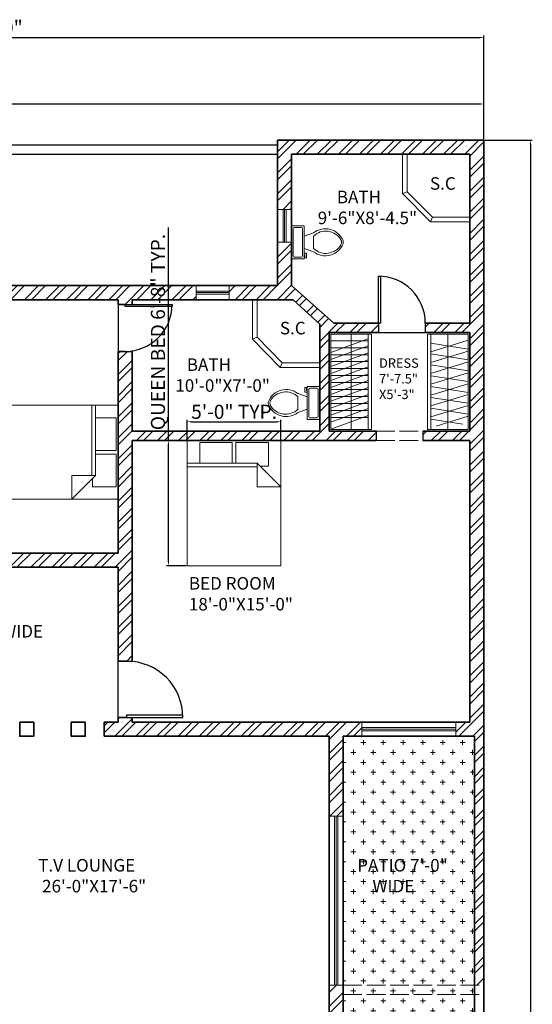
# Model space of a CAD drawing. Units: inches. Extents: x 839 to 1638, y 2998 to 4342.
# Tile 4 of 4: x 1223 to 1551, y 3713 to 4342. Entities that reach past the tile are written whole.
import ezdxf

# ---------------------------------------------------------------- set-up
doc = ezdxf.new("R2010")
doc.units = ezdxf.units.IN
doc.linetypes.add('ACAD_ISO02W100', pattern=[15, 12, -3])
for name, color, linetype, lineweight in [('A-ANNO-DIMS', 2, 'Continuous', 18), ('A-AREA-IDEN', 7, 'Continuous', 18), ('A-COLS', 7, 'Continuous', 35), ('A-DOOR', 4, 'Continuous', 25), ('A-DOOR-JAMB', 7, 'Continuous', 25), ('A-FLOR-CASE', 9, 'Continuous', 20), ('A-FLOR-CASE-PATT', 252, 'Continuous', 13), ('A-FLOR-FIXT', 9, 'Continuous', 18), ('A-FLOR-OVHD', 8, 'ACAD_ISO02W100', 18), ('A-FURN', 8, 'Continuous', 18), ('A-WALL', 7, 'Continuous', 35), ('A-WALL-OVHD', 8, 'ACAD_ISO02W100', 18), ('A-WALL-PATT', 252, 'Continuous', 13), ('C-PROP', 7, 'Continuous', 30)]:
    doc.layers.add(name, color=color, linetype=linetype, lineweight=lineweight)
doc.layers.add('A-GLAZ', color=244, linetype='Continuous', lineweight=20, true_color=0x991b1e)
doc.layers.add('L-SITE-PATT', color=116, linetype='Continuous', lineweight=13, true_color=0x136734)
doc.styles.get("Standard").update_dxf_attribs({"font": 'arial.ttf'})
doc.dimstyles.new('ISO-25', dxfattribs={"dimtxt": 9, "dimasz": 2.5, "dimexe": 1.25, "dimexo": 0.625, "dimtad": 1, "dimlunit": 3, "dimtxsty": 'Standard', "dimcen": 2.5, "dimadec": 0, "dimazin": 0, "dimtfac": 1, "dimtmove": 0, "dimatfit": 3, "dimfxl": 1, "dimarcsym": 0})

# ---------------------------------------------------------------- blocks, each defined once
blk = doc.blocks.new('*U4')
for p, q in [((0, 0), (0, 6)), ((40, 0), (40, 6))]:
    blk.add_line(p, q)
blk.add_lwpolyline([(0, 0), (0, -40), (1.75, -40), (1.75, 0)], close=True)
blk.add_arc((0, 0), 40, 270, 0)
blk = doc.blocks.new('*U8')
for p, q in [((0, 0), (0, -6)), ((40, 0), (40, -6))]:
    blk.add_line(p, q)
blk.add_lwpolyline([(0, 0), (0, 40), (1.75, 40), (1.75, 0)], close=True)
blk.add_arc((0, 0), 40, 360, 90)
blk = doc.blocks.new('Bed - Queen')
for p, q in [((0, -80.00003), (0, 0)), ((0, 0), (59.99999, 0)), ((59.99999, 0), (59.99999, -80.00003)), ((7.99999, -1.2), (28.79998, -1.2)), ((7.99999, -14.4), (7.99999, -1.2)), ((28.79998, -1.2), (28.79998, -14.4)), ((31.19999, -1.2), (51.99999, -1.2)), ((31.19999, -14.4), (31.19999, -1.2)), ((51.99999, -1.2), (51.99999, -16.4)), ((0, -14.4), (44.8, -14.4)), ((44.8, -16.8), (0, -16.8)), ((59.99999, -29.6), (44.8, -14.4)), ((44.8, -14.4), (44.8, -29.6)), ((51.99999, -16.4), (46.79936, -16.4)), ((44.8, -29.6), (59.99999, -29.6)), ((59.99999, -80.00003), (0, -80.00003))]:
    blk.add_line(p, q)
blk = doc.blocks.new('*U15')
for p, q in [((9.5, -6), (9.5, -2)), ((-10, -8.5), (-8, -8.5)), ((-10, -9.5), (-10, -8.5)), ((-7, -9.5), (-10, -9.5)), ((-8, -8.5), (-8, -8)), ((-7, -8), (-7, -9.5)), ((-4, -8), (-6, -14)), ((4, -8), (6, -14)), ((4, -14), (-4, -14))]:
    blk.add_line(p, q)
blk.add_lwpolyline([(10.5, -8), (10.5, 0), (-10.5, 0), (-10.5, -8)], close=True)
for points in [[(-9.5, -2), (-9.5, -6)], [(8.5, -1), (-8.5, -1)], [(-8.5, -7), (8.5, -7)]]:
    blk.add_lwpolyline(points)
for centre, radius, start, end in [((-8.62, -1.88), 0.884, 81.8699, 188.1301), ((-8.62, -6.12), 0.884, 171.8699, 278.1301), ((8.62, -1.88), 0.884, 351.8699, 98.1301), ((8.62, -6.12), 0.884, 261.8699, 8.1301), ((3.52, -21.58), 12.17, 141.46911, 247.97143), ((4.2, -21.82), 11.33, 136.36773, 238.94682), ((-3.52, -21.58), 12.17, 292.02843, 38.53071), ((-4.2, -21.82), 11.33, 301.05301, 43.63209), ((0, -27.88), 4, 245.73182, 294.26817), ((0, -29), 4, 254.86053, 285.13947)]:
    blk.add_arc(centre, radius, start, end)
blk = doc.blocks.new('*D20')
at = {"layer": 'A-ANNO-DIMS', "color": 0, "lineweight": -2, "transparency": 16777216}
for p, q in [((839.17, 4265.09), (839.17, 4289.16)), ((841.67, 4287.91), (1517.67, 4287.91)), ((1520.17, 4265.46), (1520.17, 4289.16))]:
    blk.add_line(p, q, dxfattribs=at)
at = {"layer": 'A-ANNO-DIMS', "color": 0, "transparency": 16777216}
for points in [[(841.67, 4288.33), (841.67, 4287.5), (839.17, 4287.91)], [(1517.67, 4288.33), (1517.67, 4287.5), (1520.17, 4287.91)]]:
    blk.add_solid(points, dxfattribs=at)
at = {"layer": 'Defpoints', "color": 0, "transparency": 16777216}
for p in [(1520.17, 4287.91), (839.17, 4264.46), (1520.17, 4264.84)]:
    blk.add_point(p, dxfattribs=at)
at = {"layer": 'A-ANNO-DIMS', "color": 0, "transparency": 16777216, "insert": (1179.67, 4293.13), "char_height": 9, "attachment_point": 5}
blk.add_mtext('56\'-9"', dxfattribs=at)
blk = doc.blocks.new('*D21')
at = {"layer": 'A-ANNO-DIMS', "color": 0, "lineweight": -2, "transparency": 16777216}
for p, q in [((1520.79, 4264.84), (1551.14, 4264.84)), ((1549.89, 4262.34), (1549.89, 3064.34)), ((1520.79, 3061.84), (1551.14, 3061.84))]:
    blk.add_line(p, q, dxfattribs=at)
at = {"layer": 'A-ANNO-DIMS', "color": 0, "transparency": 16777216}
for points in [[(1549.48, 4262.34), (1550.31, 4262.34), (1549.89, 4264.84)], [(1549.48, 3064.34), (1550.31, 3064.34), (1549.89, 3061.84)]]:
    blk.add_solid(points, dxfattribs=at)
at = {"layer": 'Defpoints', "color": 0, "transparency": 16777216}
for p in [(1520.17, 4264.84), (1520.17, 3061.84), (1549.89, 3061.84)]:
    blk.add_point(p, dxfattribs=at)
at = {"layer": 'A-ANNO-DIMS', "color": 0, "transparency": 16777216, "insert": (1544.67, 3663.34), "char_height": 9, "attachment_point": 5, "rotation": 90}
blk.add_mtext('100\'-3"', dxfattribs=at)
blk = doc.blocks.new('WIN-60x9')
for p, q in [((3.5, 60), (3.5, 0)), ((4.5, 60), (4.5, 0)), ((5.5, 60), (5.5, 0))]:
    blk.add_line(p, q)
blk.add_lwpolyline([(9, 60), (9, 0), (0, 0), (0, 60)], close=True)
blk = doc.blocks.new('WIN-21x9')
for p, q in [((0, 5.5), (21, 5.5)), ((0, 4.5), (21, 4.5)), ((0, 3.5), (21, 3.5))]:
    blk.add_line(p, q)
blk.add_lwpolyline([(0, 9), (21, 9), (21, 0), (0, 0)], close=True)
blk = doc.blocks.new('POST-9x9')
blk.add_lwpolyline([(0, 9), (9, 9), (9, 0), (0, 0)], close=True)
blk = doc.blocks.new('SHOWER-CORNER')
for p, q in [((40.25, 43.12), (40.25, 19.12)), ((43.25, 43.12), (43.25, 17.87)), ((24, 3), (40.25, 19.12)), ((40.25, 19.12), (43.25, 17.87)), ((25.23, 0), (43.25, 17.87)), ((0, 3), (24, 3)), ((0, 0), (25.23, 0)), ((24, 3), (25.23, 0))]:
    blk.add_line(p, q)
blk = doc.blocks.new('*D34')
at = {"layer": 'A-ANNO-DIMS', "color": 0, "lineweight": -2, "transparency": 16777216}
for p, q in [((1318.34, 4072.84), (1318.34, 4208.98)), ((1329.72, 4072.84), (1317.09, 4072.84)), ((1318.34, 3995.34), (1318.34, 4070.34)), ((1329.72, 3992.84), (1317.09, 3992.84))]:
    blk.add_line(p, q, dxfattribs=at)
at = {"layer": 'A-ANNO-DIMS', "color": 0, "transparency": 16777216}
for points in [[(1317.93, 4070.34), (1318.76, 4070.34), (1318.34, 4072.84)], [(1317.93, 3995.34), (1318.76, 3995.34), (1318.34, 3992.84)]]:
    blk.add_solid(points, dxfattribs=at)
at = {"layer": 'Defpoints', "color": 0, "transparency": 16777216}
for p in [(1318.34, 4072.84), (1330.34, 4072.84), (1330.34, 3992.84)]:
    blk.add_point(p, dxfattribs=at)
at = {"layer": 'A-ANNO-DIMS', "color": 0, "transparency": 16777216, "insert": (1312.79, 4142.16), "char_height": 9, "attachment_point": 5, "rotation": 90}
blk.add_mtext('QUEEN BED 6\'-8" TYP.', dxfattribs=at)
blk = doc.blocks.new('*D35')
at = {"layer": 'A-ANNO-DIMS', "color": 0, "lineweight": -2, "transparency": 16777216}
for p, q in [((1330.34, 4073.46), (1330.34, 4086.09)), ((1332.84, 4084.84), (1387.84, 4084.84)), ((1390.34, 4073.46), (1390.34, 4086.09))]:
    blk.add_line(p, q, dxfattribs=at)
at = {"layer": 'A-ANNO-DIMS', "color": 0, "transparency": 16777216}
for points in [[(1332.84, 4085.25), (1332.84, 4084.42), (1330.34, 4084.84)], [(1387.84, 4085.25), (1387.84, 4084.42), (1390.34, 4084.84)]]:
    blk.add_solid(points, dxfattribs=at)
at = {"layer": 'Defpoints', "color": 0, "transparency": 16777216}
for p in [(1390.34, 4084.84), (1330.34, 4072.84), (1390.34, 4072.84)]:
    blk.add_point(p, dxfattribs=at)
at = {"layer": 'A-ANNO-DIMS', "color": 0, "transparency": 16777216, "insert": (1360.34, 4090.06), "char_height": 9, "attachment_point": 5}
blk.add_mtext('5\'-0" TYP.', dxfattribs=at)
blk = doc.blocks.new('*D50')
at = {"layer": 'A-ANNO-DIMS', "color": 0, "lineweight": -2, "transparency": 16777216}
for p, q in [((896.17, 4172.46), (896.17, 4331.69)), ((898.67, 4330.44), (1517.67, 4330.44)), ((1520.17, 4265.46), (1520.17, 4331.69))]:
    blk.add_line(p, q, dxfattribs=at)
at = {"layer": 'A-ANNO-DIMS', "color": 0, "transparency": 16777216}
for points in [[(898.67, 4330.85), (898.67, 4330.02), (896.17, 4330.44)], [(1517.67, 4330.85), (1517.67, 4330.02), (1520.17, 4330.44)]]:
    blk.add_solid(points, dxfattribs=at)
at = {"layer": 'Defpoints', "color": 0, "transparency": 16777216}
for p in [(1520.17, 4330.44), (1520.17, 4264.84), (896.17, 4171.84)]:
    blk.add_point(p, dxfattribs=at)
at = {"layer": 'A-ANNO-DIMS', "color": 0, "transparency": 16777216, "insert": (1208.17, 4335.66), "char_height": 9, "attachment_point": 5}
blk.add_mtext('52\'-0"', dxfattribs=at)

msp = doc.modelspace()

# ---------------------------------------------------------------- hatches: boundary and pattern name
at = {"layer": 'A-FLOR-CASE-PATT'}
h = msp.add_hatch(dxfattribs=at)
h.set_pattern_fill('ANSI31', color=256, scale=1.319035, angle=-24.97004, style=0)
h.paths.add_polyline_path([(1422.169, 4133.326), (1422.169, 4079.836), (1446.169, 4088.585), (1446.169, 4137.618), (1442.767, 4140.836)])
h = msp.add_hatch(dxfattribs=at)
h.set_pattern_fill('ANSI31', color=256, scale=2.089406, angle=-28.02867, style=0)
h.paths.add_polyline_path([(1510.169, 4140.836), (1486.169, 4133.511), (1486.169, 4084.96), (1492.105, 4079.836), (1510.169, 4085.348)])
h = msp.add_hatch(dxfattribs=at)
h.set_pattern_fill('ANSI31', color=256, scale=1.403955, angle=-45, style=0)
h.paths.add_polyline_path([(1422.169, 4084.293), (1446.169, 4084.293), (1446.169, 4137.784), (1422.169, 4137.784)])
h = msp.add_hatch(dxfattribs=at)
h.set_pattern_fill('ANSI31', color=256, scale=2.157832, angle=126.0313, style=0)
h.paths.add_polyline_path([(1510.169, 4133.9), (1486.169, 4137.688), (1486.169, 4082.2), (1501.151, 4079.836), (1510.169, 4085.348)])
at = {"layer": 'A-WALL-PATT'}
h = msp.add_hatch(dxfattribs=at)
h.set_pattern_fill('ANSI32', color=256)
h.paths.add_polyline_path([(1440.674, 3673.836), (1430.169, 3673.836), (1430.169, 3724.836), (1421.169, 3724.836), (1421.169, 3673.836), (1209.669, 3673.836), (1209.669, 3670.236), (1209.669, 3664.836), (1247.169, 3664.836), (1247.169, 3661.836), (1252.569, 3661.836), (1256.169, 3661.836), (1256.169, 3664.836), (1440.674, 3664.836)])
h.paths.add_polyline_path([(1137.669, 3673.836), (1100.169, 3673.836), (1100.169, 3733.836), (1091.169, 3733.836), (1067.169, 3733.836), (1067.169, 3727.836), (1091.169, 3727.836), (1091.169, 3640.836), (971.169, 3640.836), (971.169, 3694.836), (962.169, 3694.836), (962.169, 3640.836), (896.169, 3640.836), (896.169, 3628.836), (905.169, 3628.836), (905.169, 3631.836), (1091.169, 3631.836), (1091.169, 3628.836), (1100.169, 3628.836), (1100.169, 3664.836), (1137.669, 3664.836)])
h.paths.add_polyline_path([(1256.169, 3625.836), (1247.169, 3625.836), (1247.169, 3491.75), (1237.967, 3478.332), (1245.508, 3473.161), (1247.169, 3475.836), (1520.169, 3475.836), (1520.169, 3595.836), (1504.368, 3595.836), (1504.368, 3586.836), (1511.169, 3586.836), (1511.169, 3484.836), (1439.169, 3484.836), (1439.169, 3550.955), (1415.169, 3550.955), (1415.169, 3586.836), (1418.169, 3586.836), (1418.169, 3595.836), (1406.169, 3595.836), (1406.169, 3544.955), (1433.169, 3544.955), (1433.169, 3484.836), (1406.169, 3484.836), (1256.169, 3484.836)])
h.paths.add_polyline_path([(1483.368, 3595.836), (1472.169, 3595.836), (1472.169, 3600.336), (1463.169, 3600.336), (1463.169, 3595.836), (1448.169, 3595.836), (1448.169, 3586.836), (1483.368, 3586.836)], flags=17)
h.paths.add_polyline_path([(1220.169, 3432.336), (1210.822, 3438.745), (1206.427, 3432.336), (1179.669, 3432.336), (1179.669, 3423.336), (1211.169, 3423.336), (1211.169, 3298.836), (1367.169, 3298.836), (1367.169, 3307.836), (1220.169, 3307.836)])
h.paths.add_polyline_path([(1041.669, 3532.086), (1058.169, 3532.086), (1058.169, 3541.086), (1032.669, 3541.086), (1032.669, 3432.336), (905.169, 3432.336), (905.169, 3470.704), (896.169, 3470.704), (896.169, 3423.336), (1055.555, 3423.336), (1055.555, 3432.336), (1041.669, 3432.336)])
h.paths.add_polyline_path([(1100.169, 3592.836), (1091.169, 3592.836), (1091.169, 3541.086), (1088.169, 3541.086), (1088.169, 3532.086), (1091.169, 3532.086), (1091.169, 3432.336), (1076.555, 3432.336), (1076.555, 3423.336), (1100.169, 3423.336), (1107.669, 3423.336), (1107.669, 3432.336), (1100.169, 3432.336)])
h.paths.add_polyline_path([(905.169, 3592.836), (896.169, 3592.836), (896.169, 3566.704), (905.169, 3566.704)])
h.paths.add_polyline_path([(905.169, 3763.836), (896.169, 3763.836), (896.169, 3727.836), (962.169, 3727.836), (962.169, 3724.836), (971.169, 3724.836), (971.169, 3727.836), (1031.169, 3727.836), (1031.169, 3733.836), (905.169, 3733.836)])
h.paths.add_polyline_path([(1109.169, 3892.836), (1100.169, 3892.836), (1100.169, 3895.836), (1091.169, 3895.836), (1091.169, 3886.836), (905.169, 3886.836), (905.169, 3937.836), (896.169, 3937.836), (896.169, 3847.836), (905.169, 3847.836), (905.169, 3877.836), (1091.169, 3877.836), (1091.169, 3859.836), (1100.169, 3859.836), (1100.169, 3883.836), (1109.169, 3883.836)])
h.paths.add_polyline_path([(905.169, 4162.836), (962.764, 4162.836), (962.764, 4171.836), (896.169, 4171.836), (896.169, 3997.836), (905.169, 3997.836), (905.169, 4048.836), (1010.169, 4048.836), (1010.169, 4054.836), (1007.169, 4054.836), (1007.169, 4057.836), (1001.169, 4057.836), (1001.169, 4054.836), (905.169, 4054.836)])
h.paths.add_polyline_path([(1152.669, 4171.836), (983.764, 4171.836), (983.764, 4162.836), (1001.169, 4162.836), (1001.169, 4087.836), (1007.169, 4087.836), (1007.169, 4162.836), (1073.169, 4162.836), (1073.169, 4054.836), (1046.169, 4054.836), (1046.169, 4048.836), (1091.169, 4048.836), (1091.169, 3931.836), (1100.169, 3931.836), (1100.169, 3991.836), (1103.169, 3991.836), (1103.169, 4000.836), (1100.169, 4000.836), (1100.169, 4054.836), (1079.169, 4054.836), (1079.169, 4162.836), (1152.669, 4162.836)])
h.paths.add_polyline_path([(1336.119, 4171.836), (1212.669, 4171.836), (1212.669, 4162.836), (1286.169, 4162.836), (1286.169, 4159.836), (1295.169, 4159.836), (1295.169, 4162.836), (1336.119, 4162.836)], flags=17)
h.paths.add_polyline_path([(1295.169, 4129.836), (1286.169, 4129.836), (1286.169, 4000.836), (1139.169, 4000.836), (1139.169, 3991.836), (1286.169, 3991.836), (1286.169, 3931.836), (1295.169, 3931.836), (1295.169, 4072.836), (1451.169, 4072.836), (1451.169, 4078.836), (1421.169, 4078.836), (1421.169, 4141.836), (1452.669, 4141.836), (1452.669, 4147.836), (1424.169, 4147.836), (1397.169, 4171.836), (1397.169, 4199.532), (1388.169, 4199.532), (1388.169, 4171.836), (1357.119, 4171.836), (1357.119, 4162.836), (1398.069, 4162.836), (1415.169, 4147.29), (1415.169, 4078.836), (1295.169, 4078.836)])
h.paths.add_polyline_path([(1442.169, 3892.836), (1295.169, 3892.836), (1295.169, 3895.836), (1286.169, 3895.836), (1286.169, 3892.836), (1277.169, 3892.836), (1277.169, 3883.836), (1421.169, 3883.836), (1421.169, 3832.836), (1430.169, 3832.836), (1430.169, 3883.836), (1442.169, 3883.836)])
h.paths.add_polyline_path([(1520.169, 4264.836), (1388.169, 4264.836), (1388.169, 4220.532), (1397.169, 4220.532), (1397.169, 4255.836), (1511.169, 4255.836), (1511.169, 4147.836), (1482.669, 4147.836), (1482.669, 4141.836), (1511.169, 4141.836), (1511.169, 4078.836), (1481.169, 4078.836), (1481.169, 4072.836), (1511.169, 4072.836), (1511.169, 3892.836), (1502.169, 3892.836), (1502.169, 3883.836), (1514.169, 3883.836), (1514.169, 3724.836), (1520.169, 3724.836)])
h.paths.add_polyline_path([(1319.528, 4099.601), (1381.705, 4099.601), (1381.705, 4129.453), (1319.528, 4129.453)], flags=25)
at = {"layer": 'L-SITE-PATT'}
h = msp.add_hatch(dxfattribs=at)
h.set_pattern_fill('CROSS', color=256)
h.paths.add_polyline_path([(1514.169, 3883.836), (1430.169, 3883.836), (1430.169, 3724.836), (1514.169, 3724.836)])
h.paths.add_polyline_path([(1514.169, 3718.836), (1430.169, 3718.836), (1430.169, 3673.836), (1514.169, 3673.836)])
h.paths.add_polyline_path([(1514.169, 3724.836), (1430.169, 3724.836), (1430.169, 3718.836), (1514.169, 3718.836)])
h.paths.add_polyline_path([(1436.251, 3779.553), (1499.144, 3779.553), (1499.144, 3809.372), (1436.251, 3809.372)], flags=24)

# ---------------------------------------------------------------- linework, layer by layer
at = {"layer": 'A-DOOR'}
for p, q in [((1286.169, 4159.836), (1286.169, 4129.836)), ((1452.669, 4141.836), (1482.669, 4141.836)), ((1286.169, 3895.836), (1286.169, 3931.836))]:
    msp.add_line(p, q, dxfattribs=at)
at = {"layer": 'A-DOOR-JAMB'}
for p, q in [((1286.169, 4159.836), (1295.169, 4159.836)), ((1452.669, 4147.836), (1452.669, 4141.836)), ((1482.669, 4147.836), (1482.669, 4141.836)), ((1286.169, 4129.836), (1295.169, 4129.836)), ((1451.169, 4078.836), (1451.169, 4072.836)), ((1481.169, 4078.836), (1481.169, 4072.836)), ((1286.169, 3931.836), (1295.169, 3931.836)), ((1286.169, 3895.836), (1295.169, 3895.836))]:
    msp.add_line(p, q, dxfattribs=at)
at = {"layer": 'A-FLOR-CASE'}
for p, q in [((1422.169, 4140.836), (1422.169, 4079.836)), ((1422.169, 4140.836), (1448.169, 4140.836)), ((1435.169, 4140.836), (1435.169, 4079.836)), ((1446.169, 4140.836), (1446.169, 4079.836)), ((1448.169, 4140.836), (1448.169, 4079.836)), ((1484.169, 4140.836), (1510.169, 4140.836)), ((1484.169, 4140.836), (1484.169, 4079.836)), ((1486.169, 4140.836), (1486.169, 4079.836)), ((1497.169, 4079.836), (1497.169, 4140.836)), ((1510.169, 4140.836), (1510.169, 4079.836)), ((1422.169, 4079.836), (1448.169, 4079.836)), ((1484.169, 4079.836), (1510.169, 4079.836))]:
    msp.add_line(p, q, dxfattribs=at)
at = {"layer": 'A-FLOR-OVHD'}
for p, q in [((1430.169, 3724.836), (1520.169, 3724.836)), ((1430.169, 3718.836), (1520.169, 3718.836))]:
    msp.add_line(p, q, dxfattribs=at)
at = {"layer": 'A-GLAZ'}
for p, q in [((1424.669, 3832.836), (1424.669, 3724.836)), ((1425.669, 3832.836), (1425.669, 3724.836)), ((1426.669, 3832.836), (1426.669, 3724.836))]:
    msp.add_line(p, q, dxfattribs=at)
msp.add_lwpolyline([(1430.169, 3832.836), (1430.169, 3724.836), (1421.169, 3724.836), (1421.169, 3832.836)], close=True, dxfattribs=at)
at = {"layer": 'A-WALL'}
for p, q in [((1388.169, 4264.836), (1388.169, 4171.836)), ((1388.169, 4264.836), (1520.169, 4264.836)), ((1520.169, 4264.836), (1520.169, 3703.057)), ((1397.169, 4255.836), (1397.169, 4171.836)), ((1397.169, 4255.836), (1511.169, 4255.836)), ((1511.169, 4255.836), (1511.169, 4147.836)), ((896.169, 4171.836), (1388.169, 4171.836)), ((1397.169, 4171.836), (1424.169, 4147.836)), ((1079.169, 4162.836), (1286.169, 4162.836)), ((1286.169, 4162.836), (1286.169, 4159.836)), ((1295.169, 4162.836), (1295.169, 4159.836)), ((1295.169, 4162.836), (1398.069, 4162.836)), ((1398.069, 4162.836), (1415.169, 4147.29)), ((1415.169, 4147.29), (1415.169, 4078.836)), ((1424.169, 4147.836), (1452.669, 4147.836)), ((1482.669, 4147.836), (1511.169, 4147.836)), ((1421.169, 4141.836), (1452.669, 4141.836)), ((1421.169, 4141.836), (1421.169, 4078.836)), ((1482.669, 4141.836), (1511.169, 4141.836)), ((1511.169, 4141.836), (1511.169, 4078.836)), ((1286.169, 4129.836), (1286.169, 4000.836)), ((1295.169, 4129.836), (1295.169, 4078.836)), ((1295.169, 4078.836), (1415.169, 4078.836)), ((1421.169, 4078.836), (1451.169, 4078.836)), ((1481.169, 4078.836), (1511.169, 4078.836)), ((1295.169, 4072.836), (1451.169, 4072.836)), ((1295.169, 4072.836), (1295.169, 3931.836)), ((1481.169, 4072.836), (1511.169, 4072.836)), ((1511.169, 4072.836), (1511.169, 3892.836)), ((1139.169, 4000.836), (1286.169, 4000.836)), ((1139.169, 3991.836), (1286.169, 3991.836)), ((1286.169, 3991.836), (1286.169, 3931.836)), ((1286.169, 3895.836), (1286.169, 3892.836)), ((1295.169, 3895.836), (1295.169, 3892.836)), ((1277.169, 3892.836), (1277.169, 3883.836)), ((1286.169, 3892.836), (1277.169, 3892.836)), ((1295.169, 3892.836), (1511.169, 3892.836)), ((1277.169, 3883.836), (1421.169, 3883.836)), ((1421.169, 3883.836), (1421.169, 3673.836)), ((1430.169, 3883.836), (1430.169, 3673.836)), ((1430.169, 3883.836), (1514.169, 3883.836)), ((1514.169, 3883.836), (1514.169, 3595.836))]:
    msp.add_line(p, q, dxfattribs=at)
at = {"layer": 'A-WALL-OVHD'}
for p, q in [((1451.169, 4078.836), (1481.169, 4078.836)), ((1451.169, 4072.836), (1481.169, 4072.836))]:
    msp.add_line(p, q, dxfattribs=at)
at = {"layer": 'C-PROP'}
for p, q in [((839.169, 4261.836), (1388.169, 4261.836)), ((845.169, 4255.836), (1388.169, 4255.836))]:
    msp.add_line(p, q, dxfattribs=at)

# ---------------------------------------------------------------- block references
at = {"layer": 'A-COLS'}
for p in [(1223.169, 3883.836), (1256.169, 3883.836)]:
    msp.add_blockref('POST-9x9', p, dxfattribs=at)
at = {"layer": 'A-DOOR', "xscale": 0.7499999999999982, "yscale": 0.7499999999999982, "zscale": 0.7499999999999982}
msp.add_blockref('*U8', (1452.669, 4147.836), dxfattribs=at)
at = {"layer": 'A-DOOR'}
for name, p, xscale, yscale, zscale, rotation in [('*U8', (1290.669, 4159.836), 0.7499999999999982, 0.7499999999999982, 0.7499999999999982, 270), ('*U4', (1291.569, 3895.836), 0.900000000000001, 0.900000000000001, 0.900000000000001, 90)]:
    msp.add_blockref(name, p, dxfattribs=dict(at, xscale=xscale, yscale=yscale, zscale=zscale, rotation=rotation))
at = {"layer": 'A-FLOR-FIXT'}
for name, p, rotation in [('SHOWER-CORNER', (1468.051, 4255.835), 269.9999999999998), ('*U15', (1397.169, 4199.532), 89.99999999999999), ('SHOWER-CORNER', (1372.051, 4162.835), 269.9999999999991), ('*U15', (1415.169, 4096.804), 270)]:
    msp.add_blockref(name, p, dxfattribs=dict(at, rotation=rotation))
at = {"layer": 'A-FURN', "rotation": 270}
msp.add_blockref('Bed - Queen', (1286.169, 4095.336), dxfattribs=at)
at = {"layer": 'A-FURN'}
msp.add_blockref('Bed - Queen', (1330.342, 4072.836), dxfattribs=at)
at = {"layer": 'A-GLAZ'}
for name, p, rotation in [('WIN-21x9', (1388.169, 4220.532), 269.9999999999986), ('WIN-60x9', (1502.168, 3883.836), 90.00000000000055)]:
    msp.add_blockref(name, p, dxfattribs=dict(at, rotation=rotation))
msp.add_blockref('WIN-21x9', (1336.118, 4162.836), dxfattribs=at)

# ---------------------------------------------------------------- texts
at = {"layer": 'A-AREA-IDEN', "attachment_point": 1}
for s, width, insert, char_height in [('S.C', 16.07573, (1485.651, 4241.113), 8), ('     BATH\\P9\'-6"X8\'-4.5"', 61.95293, (1413.851, 4232.455), 8), ('S.C', 16.07573, (1389.643, 4148.682), 8), ('   BATH\\P10\'-0"X7\'-0"', 51.99955, (1322.745, 4125.336), 8), ('DRESS\\P7\'-7.5"\\PX5\'-3"', 31.7046, (1453.077, 4125.336), 6), ('BED ROOM\\P18\'-0"X15\'-0"', 66.18672, (1331.405, 3985.569), 8), ('LOBBY 5\'-7.5" WIDE', 104.90723, (1139.169, 3954.925), 8), ('T.V LOUNGE \\P 26\'-0"X17\'-6"', 70.597, (1235.057, 3805.397), 8), ('PATIO 7\'-0" \\P    WIDE', 59.82661, (1439.113, 3805.397), 8)]:
    msp.add_mtext_dynamic_manual_height_columns(s, width=width, gutter_width=12.5, heights=[0], dxfattribs=dict(at, insert=insert, char_height=char_height))

# ---------------------------------------------------------------- dimensions: what is measured, and where the dimension line sits
at = {"layer": 'A-ANNO-DIMS'}
for base, p1, override, picture, middle in [((1520.169, 4330.436), (896.169, 4171.836), {"dimdec": 1, "dimlfac": 1, "dimrnd": 0, "dimzin": 1, "dimdsep": 46, "dimlunit": 4, "dimfrac": 2}, '*D50', (1208.169, 4335.656)), ((1520.169, 4287.912), (839.169, 4264.461), {"dimclrd": 0, "dimclre": 0, "dimclrt": 0}, '*D20', (1179.669, 4293.132))]:
    dim = msp.add_linear_dim(base=base, p1=p1, p2=(1520.169, 4264.836), dimstyle='ISO-25', override=override, dxfattribs=at)
    dim.commit()
    dim.dimension.update_dxf_attribs({"geometry": picture, "text_midpoint": middle})
dim = msp.add_linear_dim(base=(1549.893, 3061.836), p1=(1520.169, 4264.836), p2=(1520.169, 3061.836), angle=90, dimstyle='ISO-25', override={"dimclrd": 0, "dimclre": 0, "dimclrt": 0}, dxfattribs=at)
dim.commit()
dim.dimension.update_dxf_attribs({"geometry": '*D21', "text_midpoint": (1544.67, 3663.336)})
dim = msp.add_linear_dim(base=(1318.342, 4072.836), p1=(1330.342, 3992.836), p2=(1330.342, 4072.836), angle=90, text='QUEEN BED <> TYP.', dimstyle='ISO-25', override={"dimdec": 1, "dimlfac": 1, "dimrnd": 0, "dimzin": 1, "dimdsep": 46, "dimlunit": 4, "dimfrac": 2}, dxfattribs=at)
dim.commit()
dim.dimension.update_dxf_attribs({"geometry": '*D34', "text_midpoint": (1312.787, 4142.156)})
dim = msp.add_linear_dim(base=(1390.342, 4084.836), p1=(1330.342, 4072.836), p2=(1390.342, 4072.836), text='<> TYP.', dimstyle='ISO-25', override={"dimdec": 1, "dimlfac": 1, "dimrnd": 0, "dimzin": 1, "dimdsep": 46, "dimlunit": 4, "dimfrac": 2}, dxfattribs=at)
dim.commit()
dim.dimension.update_dxf_attribs({"geometry": '*D35', "text_midpoint": (1360.342, 4090.056)})

doc.saveas('drawing.dxf')
